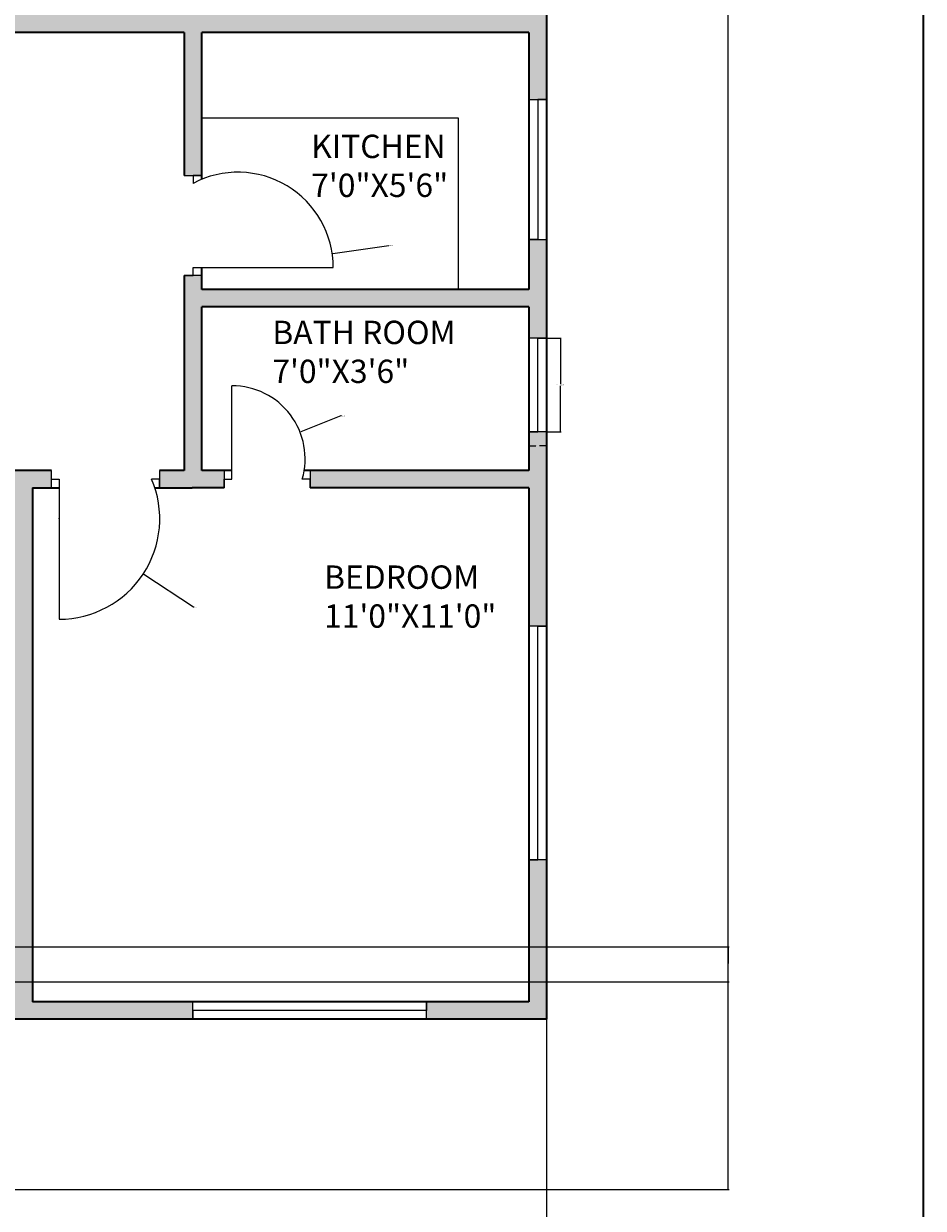
# Model space of a CAD drawing. Units: inches. Extents: x 2314 to 3223, y 1382 to 2735.
# Tile 5 of 14: x 2992 to 3223, y 1560 to 1864. Entities that reach past the tile are written whole.
import ezdxf

# ---------------------------------------------------------------- set-up
doc = ezdxf.new("R2010")
doc.units = ezdxf.units.IN
for name, color, linetype, lineweight in [('A-ANNO-DIMS', 2, 'Continuous', 18), ('A-ANNO-TTLB', 7, 'Continuous', 35), ('A-AREA-IDEN', 7, 'Continuous', 18), ('A-DOOR', 3, 'Continuous', 18), ('A-FLOR-FIXT', 8, 'Continuous', 18), ('A-GLAZ', 4, 'Continuous', 18), ('A-WALL', 7, 'Continuous', 35)]:
    doc.layers.add(name, color=color, linetype=linetype, lineweight=lineweight)
doc.layers.add('A-WALL-PATT', color=251, linetype='Continuous', lineweight=13, true_color=0x636466)
doc.styles.get("Standard").update_dxf_attribs({"font": 'arial.ttf'})
doc.dimstyles.get("Standard").update_dxf_attribs({"dimtxt": 0.18, "dimasz": 0.18, "dimexe": 0.18, "dimexo": 0.0625, "dimgap": 0.09, "dimtad": 0, "dimtih": 1, "dimtoh": 1, "dimdec": 4, "dimzin": 0, "dimdsep": 46, "dimtxsty": 'Standard', "dimcen": 0.09, "dimadec": 0, "dimazin": 0, "dimtfac": 1, "dimtdec": 4, "dimtofl": 0, "dimtmove": 0, "dimatfit": 3, "dimfxl": 1, "dimtolj": 1, "dimtzin": 0, "dimarcsym": 0})

# ---------------------------------------------------------------- blocks, each defined once
blk = doc.blocks.new('WIN-PLAN-24')
for p, q in [((0, 24), (4.5, 24)), ((4.5, 24), (2.25, 24)), ((2.25, 24), (2.25, 0)), ((2.25, 0), (0, 0)), ((0, 0), (4.5, 0))]:
    blk.add_line(p, q)
blk = doc.blocks.new('WIN-PLAN-60')
for p, q in [((0, 4.5), (0, 0)), ((60, 2.25), (60, 4.5)), ((60, 4.5), (60, 0)), ((0, 0), (0, 2.25)), ((0, 2.25), (60, 2.25))]:
    blk.add_line(p, q)
blk = doc.blocks.new('WIN-PLAN-36')
for p, q in [((0, 36), (4.5, 36)), ((4.5, 36), (2.25, 36)), ((2.25, 36), (2.25, 0)), ((2.25, 0), (0, 0)), ((0, 0), (4.5, 0))]:
    blk.add_line(p, q)
blk = doc.blocks.new('*D13')
at = {"layer": 'A-ANNO-DIMS', "color": 0, "lineweight": -2, "transparency": 16777216}
for p, q in [((3125.96, 1783.31), (3129.67, 1783.31)), ((3129.49, 1783.13), (3129.49, 1771.49)), ((3129.49, 1759.49), (3129.49, 1771.13)), ((3125.96, 1759.31), (3129.67, 1759.31))]:
    blk.add_line(p, q, dxfattribs=at)
at = {"layer": 'A-ANNO-DIMS', "color": 0, "transparency": 16777216}
for points in [[(3129.46, 1783.13), (3129.52, 1783.13), (3129.49, 1783.31)], [(3129.46, 1759.49), (3129.52, 1759.49), (3129.49, 1759.31)]]:
    blk.add_solid(points, dxfattribs=at)
at = {"layer": 'Defpoints', "color": 0, "transparency": 16777216}
for p in [(3125.89, 1783.31), (3125.89, 1759.31), (3129.49, 1759.31)]:
    blk.add_point(p, dxfattribs=at)
at = {"layer": 'A-ANNO-DIMS', "color": 0, "transparency": 16777216, "insert": (3129.49, 1771.31), "char_height": 0.18, "attachment_point": 5}
blk.add_mtext('\\A1;WINDOW 24 TYP.', dxfattribs=at)
blk = doc.blocks.new('*D14')
at = {"layer": 'A-ANNO-DIMS', "color": 0, "lineweight": -2, "transparency": 16777216}
for p, q in [((3121.39, 1759.25), (3121.39, 1755.53)), ((3125.89, 1759.25), (3125.89, 1755.53)), ((3121.57, 1755.71), (3123.18, 1755.71)), ((3125.71, 1755.71), (3124.1, 1755.71))]:
    blk.add_line(p, q, dxfattribs=at)
at = {"layer": 'A-ANNO-DIMS', "color": 0, "transparency": 16777216}
for points in [[(3121.57, 1755.74), (3121.57, 1755.68), (3121.39, 1755.71)], [(3125.71, 1755.74), (3125.71, 1755.68), (3125.89, 1755.71)]]:
    blk.add_solid(points, dxfattribs=at)
at = {"layer": 'Defpoints', "color": 0, "transparency": 16777216}
for p in [(3121.39, 1759.31), (3125.89, 1759.31), (3121.39, 1755.71)]:
    blk.add_point(p, dxfattribs=at)
at = {"layer": 'A-ANNO-DIMS', "color": 0, "transparency": 16777216, "insert": (3123.64, 1755.71), "char_height": 0.18, "attachment_point": 5}
blk.add_mtext('\\A1;5 TYP.', dxfattribs=at)
blk = doc.blocks.new('*D29')
at = {"layer": 'A-ANNO-DIMS', "color": 0, "lineweight": -2, "transparency": 16777216}
for p, q in [((2410.39, 1608.32), (2410.39, 1434.13)), ((3125.89, 1608.32), (3125.89, 1434.13)), ((2410.57, 1434.31), (2767.75, 1434.31)), ((3125.71, 1434.31), (2768.54, 1434.31))]:
    blk.add_line(p, q, dxfattribs=at)
at = {"layer": 'A-ANNO-DIMS', "color": 0, "transparency": 16777216}
for points in [[(2410.57, 1434.34), (2410.57, 1434.28), (2410.39, 1434.31)], [(3125.71, 1434.34), (3125.71, 1434.28), (3125.89, 1434.31)]]:
    blk.add_solid(points, dxfattribs=at)
at = {"layer": 'Defpoints', "color": 0, "transparency": 16777216}
for p in [(2410.39, 1608.38), (3125.89, 1608.38), (3125.89, 1434.31)]:
    blk.add_point(p, dxfattribs=at)
at = {"layer": 'A-ANNO-DIMS', "color": 0, "transparency": 16777216, "insert": (2768.14, 1434.31), "char_height": 0.18, "attachment_point": 5}
blk.add_mtext('\\A1;715.5', dxfattribs=at)
blk = doc.blocks.new('*D30')
at = {"layer": 'A-ANNO-DIMS', "color": 0, "lineweight": -2, "transparency": 16777216}
for p, q in [((3125.96, 2381.78), (3172.77, 2381.78)), ((3172.59, 2381.6), (3172.59, 1973.38)), ((3172.59, 1564.8), (3172.59, 1973.02)), ((2822.96, 1564.62), (3172.77, 1564.62))]:
    blk.add_line(p, q, dxfattribs=at)
at = {"layer": 'A-ANNO-DIMS', "color": 0, "transparency": 16777216}
for points in [[(3172.56, 2381.6), (3172.62, 2381.6), (3172.59, 2381.78)], [(3172.56, 1564.8), (3172.62, 1564.8), (3172.59, 1564.62)]]:
    blk.add_solid(points, dxfattribs=at)
at = {"layer": 'Defpoints', "color": 0, "transparency": 16777216}
for p in [(3125.89, 2381.78), (2822.89, 1564.62), (3172.59, 1564.62)]:
    blk.add_point(p, dxfattribs=at)
at = {"layer": 'A-ANNO-DIMS', "color": 0, "transparency": 16777216, "insert": (3172.59, 1973.2), "char_height": 0.18, "attachment_point": 5}
blk.add_mtext('\\A1;817.2', dxfattribs=at)
blk = doc.blocks.new('*D38')
at = {"layer": 'A-ANNO-DIMS', "color": 0, "lineweight": -2, "transparency": 16777216}
for p, q in [((2818.46, 1627), (3172.77, 1627)), ((3172.59, 1626.82), (3172.59, 1622.68)), ((3172.59, 1618.18), (3172.59, 1622.32)), ((2818.46, 1618), (3172.77, 1618))]:
    blk.add_line(p, q, dxfattribs=at)
at = {"layer": 'A-ANNO-DIMS', "color": 0, "transparency": 16777216}
for points in [[(3172.56, 1626.82), (3172.62, 1626.82), (3172.59, 1627)], [(3172.56, 1618.18), (3172.62, 1618.18), (3172.59, 1618)]]:
    blk.add_solid(points, dxfattribs=at)
at = {"layer": 'Defpoints', "color": 0, "transparency": 16777216}
for p in [(2818.39, 1627), (3172.59, 1627), (2818.39, 1618)]:
    blk.add_point(p, dxfattribs=at)
at = {"layer": 'A-ANNO-DIMS', "color": 0, "transparency": 16777216, "insert": (3172.59, 1622.5), "char_height": 0.18, "attachment_point": 5}
blk.add_mtext('\\A1;9', dxfattribs=at)
blk = doc.blocks.new('*D80')
at = {"layer": 'A-ANNO-DIMS', "color": 0, "lineweight": -2, "transparency": 16777216}
for p, q in [((3000.65, 1736.98), (3000.83, 1736.98)), ((3000.74, 1736.89), (3000.74, 1737.07)), ((3035.25, 1714.2), (3022.46, 1722.64)), ((3035.43, 1714.2), (3035.25, 1714.2))]:
    blk.add_line(p, q, dxfattribs=at)
at = {"layer": 'A-ANNO-DIMS', "color": 0, "transparency": 16777216}
blk.add_solid([(3022.48, 1722.67), (3022.44, 1722.62), (3022.31, 1722.74)], dxfattribs=at)
at = {"layer": 'Defpoints', "color": 0, "transparency": 16777216}
for p in [(3000.74, 1736.98), (3022.31, 1722.74)]:
    blk.add_point(p, dxfattribs=at)
at = {"layer": 'A-ANNO-DIMS', "color": 0, "transparency": 16777216, "insert": (3035.91, 1714.2), "char_height": 0.18, "attachment_point": 5}
blk.add_mtext('\\A1;R25.84', dxfattribs=at)
blk = doc.blocks.new('*D83')
at = {"layer": 'A-ANNO-DIMS', "color": 0, "lineweight": -2, "transparency": 16777216}
for p, q in [((3085.44, 1807.09), (3071.07, 1805.01)), ((3046.56, 1801.48), (3046.74, 1801.48)), ((3046.65, 1801.39), (3046.65, 1801.57))]:
    blk.add_line(p, q, dxfattribs=at)
at = {"layer": 'A-ANNO-DIMS', "color": 0, "transparency": 16777216}
blk.add_solid([(3071.06, 1805.04), (3071.07, 1804.98), (3070.89, 1804.98)], dxfattribs=at)
at = {"layer": 'Defpoints', "color": 0, "transparency": 16777216}
for p in [(3070.89, 1804.98), (3046.65, 1801.48)]:
    blk.add_point(p, dxfattribs=at)
at = {"layer": 'A-ANNO-DIMS', "color": 0, "transparency": 16777216, "insert": (3085.99, 1807.09), "char_height": 0.18, "attachment_point": 5}
blk.add_mtext('\\A1;R24.496', dxfattribs=at)
blk = doc.blocks.new('*D95')
at = {"layer": 'A-ANNO-DIMS', "color": 0, "lineweight": -2, "transparency": 16777216}
for p, q in [((3073.1, 1763.38), (3062.78, 1759.31)), ((3073.28, 1763.38), (3073.1, 1763.38)), ((3045.04, 1752.34), (3045.22, 1752.34)), ((3045.13, 1752.25), (3045.13, 1752.43))]:
    blk.add_line(p, q, dxfattribs=at)
at = {"layer": 'A-ANNO-DIMS', "color": 0, "transparency": 16777216}
blk.add_solid([(3062.77, 1759.33), (3062.79, 1759.28), (3062.61, 1759.24)], dxfattribs=at)
at = {"layer": 'Defpoints', "color": 0, "transparency": 16777216}
for p in [(3062.61, 1759.24), (3045.13, 1752.34)]:
    blk.add_point(p, dxfattribs=at)
at = {"layer": 'A-ANNO-DIMS', "color": 0, "transparency": 16777216, "insert": (3073.76, 1763.38), "char_height": 0.18, "attachment_point": 5}
blk.add_mtext('\\A1;R18.79', dxfattribs=at)

msp = doc.modelspace()

# ---------------------------------------------------------------- hatches: boundary and pattern name
at = {"layer": 'A-WALL-PATT'}
h = msp.add_hatch(color=256, dxfattribs=at)
h.dxf.hatch_style = 1
h.paths.add_polyline_path([(2443.3302, 2379.5332), (2443.3302, 2381.7832), (2410.3927, 2381.7832), (2410.3927, 2336.7008), (2414.8927, 2336.7008), (2414.8927, 2377.2832), (2443.3302, 2377.2832)])
h.paths.add_polyline_path([(2561.3645, 2379.5332), (2561.3645, 2381.7832), (2503.3302, 2381.7832), (2503.3302, 2377.2832), (2546.8927, 2377.2832), (2546.8927, 2245.2832), (2541.8787, 2245.2832), (2541.8787, 2240.7832), (2551.3927, 2240.7832), (2551.3927, 2377.2832), (2561.3645, 2377.2832)])
h.paths.add_polyline_path([(2656.0607, 2381.7832), (2597.3645, 2381.7832), (2597.3645, 2377.2832), (2617.3927, 2377.2832), (2617.3927, 2257.2832), (2584.2532, 2257.2832), (2584.2532, 2252.7832), (2625.8528, 2252.7832), (2625.8528, 2255.0332), (2625.8528, 2257.2832), (2621.8927, 2257.2832), (2621.8927, 2377.2832), (2656.0607, 2377.2832), (2656.0607, 2379.5332)])
h.paths.add_polyline_path([(2807.3418, 2381.7832), (2716.0607, 2381.7832), (2716.0607, 2377.2832), (2765.8927, 2377.2832), (2765.8927, 2257.2832), (2661.6935, 2257.2832), (2661.6935, 2252.7832), (2765.8927, 2252.7832), (2765.8927, 2146.2832), (2760.9259, 2146.2832), (2760.9259, 2141.8832), (2775.7119, 2141.8832), (2775.7119, 2146.2832), (2770.3927, 2146.2832), (2770.3927, 2252.7832), (2877.684, 2252.7832), (2877.684, 2255.0332), (2877.684, 2257.2832), (2770.3927, 2257.2832), (2770.3927, 2377.2832), (2807.3418, 2377.2832), (2807.3418, 2379.5332)])
h.paths.add_polyline_path([(2937.2118, 2381.7832), (2867.3418, 2381.7832), (2867.3418, 2377.2832), (2914.3927, 2377.2832), (2914.3927, 2257.2832), (2908.4124, 2257.2832), (2908.4124, 2252.7832), (2960.6432, 2252.7832), (2960.6432, 2255.0332), (2960.6432, 2257.2832), (2918.8927, 2257.2832), (2918.8927, 2377.2832), (2937.2118, 2377.2832)])
h.paths.add_polyline_path([(3022.1601, 2381.7832), (2973.2118, 2381.7832), (2973.2118, 2379.5332), (2973.2118, 2377.2832), (2984.8927, 2377.2832), (2984.8927, 2257.2832), (2980.0601, 2257.2832), (2980.0601, 2252.7832), (2984.8927, 2252.7832), (2984.8927, 2240.7832), (2995.668, 2240.7832), (2995.668, 2243.0332), (2995.668, 2245.2832), (2989.3927, 2245.2832), (2989.3927, 2377.2832), (3022.1601, 2377.2832), (3022.1601, 2379.5332)])
h.paths.add_polyline_path([(3125.8927, 2381.7832), (3082.1601, 2381.7832), (3082.1601, 2377.2832), (3121.3927, 2377.2832), (3121.3927, 2334.7388), (3125.8927, 2334.7388)])
h.paths.add_polyline_path([(3125.8927, 2274.7388), (3121.3927, 2274.7388), (3121.3927, 2245.2832), (3066.4832, 2245.2832), (3066.4832, 2240.7832), (3121.3927, 2240.7832), (3121.3927, 2232.1868), (3125.8927, 2232.1868)])
h.paths.add_polyline_path([(3125.8927, 2208.1868), (3121.3927, 2208.1868), (3121.3927, 2198.7832), (3037.3927, 2198.7832), (3037.3927, 2240.7832), (3041.2694, 2240.7832), (3041.2694, 2243.0332), (3041.2694, 2245.2832), (3026.8205, 2245.2832), (3026.8205, 2240.7832), (3032.8927, 2240.7832), (3032.8927, 2190.4022), (3037.3927, 2190.4022), (3037.3927, 2194.2832), (3121.3927, 2194.2832), (3121.3927, 2182.1835), (3125.8927, 2182.1835)])
h.paths.add_polyline_path([(3125.8927, 2158.1835), (3121.3927, 2158.1835), (3121.3927, 2146.2832), (3037.3927, 2146.2832), (3037.3927, 2169.3726), (3035.1427, 2169.3726), (3032.8927, 2169.3726), (3032.8927, 2146.2832), (2812.7301, 2146.2832), (2812.7301, 2144.0832), (2812.7301, 2141.8832), (2818.3927, 2141.8832), (2818.3927, 1970.1316), (2822.8927, 1970.1316), (2822.8927, 1978.8832), (2903.9846, 1978.8832), (2903.9846, 1981.1332), (2903.9846, 1983.3832), (2822.8927, 1983.3832), (2822.8927, 2115.3832), (2851.7162, 2115.3832), (2851.7162, 2117.6332), (2851.7162, 2119.8832), (2822.8927, 2119.8832), (2822.8927, 2141.8832), (3125.8927, 2141.8832)])
h.paths.add_polyline_path([(3125.8927, 2119.8832), (3081.193, 2119.8832), (3081.193, 2115.3832), (3121.3927, 2115.3832), (3121.3927, 2071.8188), (3125.8927, 2071.8188)], flags=17)
h.paths.add_polyline_path([(2989.3927, 2115.3832), (3021.193, 2115.3832), (3021.193, 2117.6332), (3021.193, 2119.8832), (2979.123, 2119.8832), (2979.123, 2115.3832), (2984.8927, 2115.3832), (2984.8927, 2019.3832), (2981.9225, 2019.3832), (2981.9225, 2014.8832), (2984.8927, 2014.8832), (2984.8927, 1983.3832), (2984.8927, 1978.8832), (2989.3927, 1978.8832), (2989.3927, 1983.3832)], flags=17)
h.paths.add_polyline_path([(2947.3927, 2115.3832), (2955.123, 2115.3832), (2955.123, 2117.6332), (2955.123, 2119.8832), (2911.7162, 2119.8832), (2911.7162, 2115.3832), (2942.8927, 2115.3832), (2942.8927, 1983.3832), (2936.7017, 1983.3832), (2936.7017, 1978.8832), (2947.3927, 1978.8832), (2947.3927, 1983.3832), (2947.3927, 2014.8832), (2960.7167, 2014.8832), (2960.7167, 2017.1332), (2960.7167, 2019.3832), (2947.3927, 2019.3832)], flags=17)
h.paths.add_polyline_path([(3037.3927, 1978.8832), (3041.8276, 1978.8832), (3041.8276, 1981.1332), (3041.8276, 1983.3832), (3025.477, 1983.3832), (3025.477, 1978.8832), (3032.8927, 1978.8832), (3032.8927, 1927.1259), (3035.1427, 1927.1259), (3037.3927, 1927.1259)])
h.paths.add_polyline_path([(3125.8927, 2011.8188), (3123.6427, 2011.8188), (3121.3927, 2011.8188), (3121.3927, 1983.3832), (3065, 1983.3832), (3065, 1978.8832), (3121.3927, 1978.8832), (3121.3927, 1970.5932), (3125.8927, 1970.5932)], flags=17)
h.paths.add_polyline_path([(2994.2341, 1983.3832), (2989.3927, 1983.3832), (2989.3927, 1978.8832), (2994.2341, 1978.8832), (2994.2341, 1981.1332)], flags=16)
h.paths.add_polyline_path([(3125.8927, 1946.5932), (3121.3927, 1946.5932), (3121.3927, 1936.8832), (3037.3927, 1936.8832), (3037.3927, 1932.3832), (3121.3927, 1932.3832), (3121.3927, 1919.825), (3125.8927, 1919.825)])
h.paths.add_polyline_path([(3125.8927, 1883.825), (3121.3927, 1883.825), (3121.3927, 1866.3832), (3037.3927, 1866.3832), (3037.3927, 1899.0954), (3035.1427, 1899.0954), (3032.8927, 1899.0954), (3032.8927, 1866.3832), (2822.8927, 1866.3832), (2822.8927, 1938.7212), (2820.6427, 1938.7212), (2818.3927, 1938.7212), (2818.3927, 1786.9239), (2822.8927, 1786.9239), (2822.8927, 1861.8832), (3032.8927, 1861.8832), (3032.8927, 1825.1023), (3037.3927, 1825.1023), (3037.3927, 1861.8832), (3121.3927, 1861.8832), (3121.3927, 1844.6765), (3125.8927, 1844.6765)])
h.paths.add_polyline_path([(3125.8927, 1808.6765), (3121.3927, 1808.6765), (3121.3927, 1795.8832), (3037.3927, 1795.8832), (3037.3927, 1799.4755), (3032.8927, 1799.4755), (3032.8927, 1749.3832), (3026.5034, 1749.3832), (3026.5034, 1744.8832), (3032.8927, 1744.8832), (3034.9255, 1744.8832), (3043.1326, 1744.8832), (3043.1326, 1747.1332), (3043.1326, 1749.3832), (3037.3927, 1749.3832), (3037.3927, 1791.3832), (3121.3927, 1791.3832), (3121.3927, 1783.3103), (3125.8927, 1783.3103)])
h.paths.add_polyline_path([(3125.8927, 1759.3103), (3121.3927, 1759.3103), (3121.3927, 1749.3832), (3065.1845, 1749.3832), (3065.1845, 1744.8832), (3121.3927, 1744.8832), (3121.3927, 1709.3573), (3125.8927, 1709.3573)])
h.paths.add_polyline_path([(3125.8927, 1649.3573), (3121.3927, 1649.3573), (3121.3927, 1612.8832), (3095.116, 1612.8832), (3095.116, 1608.3832), (3125.8927, 1608.3832)])
h.paths.add_polyline_path([(3035.116, 1612.8832), (2993.8927, 1612.8832), (2993.8927, 1744.8832), (2998.7409, 1744.8832), (2998.7409, 1749.3832), (2989.3927, 1749.3832), (2989.3927, 1744.8832), (2989.3927, 1701.3832), (2972.8226, 1701.3832), (2972.8226, 1696.8832), (2989.3927, 1696.8832), (2989.3927, 1612.8832), (2978.2225, 1612.8832), (2978.2225, 1608.3832), (3035.116, 1608.3832), (3035.116, 1610.6332)])
h.paths.add_polyline_path([(2947.3927, 1696.8832), (2950.7566, 1696.8832), (2950.7566, 1699.1332), (2950.7566, 1701.3832), (2947.3927, 1701.3832), (2947.3927, 1744.8832), (2947.3927, 1749.3832), (2937.649, 1749.3832), (2937.649, 1744.8832), (2942.8927, 1744.8832), (2942.8927, 1612.8832), (2907.783, 1612.8832), (2907.783, 1608.3832), (2954.2225, 1608.3832), (2954.2225, 1610.6332), (2954.2225, 1612.8832), (2947.3927, 1612.8832)])
h.paths.add_polyline_path([(2822.8927, 1744.8832), (2905.3491, 1744.8832), (2905.3491, 1747.1332), (2905.3491, 1749.3832), (2822.8927, 1749.3832), (2822.8927, 1756.9185), (2818.3927, 1756.9185), (2818.3927, 1612.8832), (2818.3927, 1569.1205), (2722.3927, 1569.1205), (2722.3927, 1612.8832), (2722.3927, 1756.9185), (2717.8927, 1756.9185), (2717.8927, 1750.0143), (2633.6297, 1750.0143), (2633.6437, 1745.2665), (2717.8927, 1745.5143), (2717.8927, 1612.8832), (2689.8467, 1612.8832), (2689.8467, 1608.3832), (2717.8927, 1608.3832), (2717.8927, 1564.6205), (2722.3927, 1564.6205), (2822.8927, 1564.6205), (2822.8927, 1569.1205), (2822.8927, 1608.3832), (2847.783, 1608.3832), (2847.783, 1610.6332), (2847.783, 1612.8832), (2822.8927, 1612.8832)])
h.paths.add_polyline_path([(2629.8467, 1612.8832), (2597.8927, 1612.8832), (2597.8927, 1744.8832), (2597.8927, 1745.1613), (2601.5887, 1745.1721), (2601.5816, 1747.5932), (2601.5745, 1750.0143), (2593.3927, 1750.0143), (2593.3927, 1744.8832), (2593.3927, 1713.3832), (2589.7588, 1713.3832), (2589.7588, 1708.8832), (2593.3927, 1708.8832), (2593.3927, 1612.8832), (2582.3793, 1612.8832), (2582.3793, 1608.3832), (2629.8467, 1608.3832), (2629.8467, 1610.6332)])
h.paths.add_polyline_path([(2551.3927, 1708.8832), (2567.6776, 1708.8832), (2567.6776, 1711.1332), (2567.6776, 1713.3832), (2551.3927, 1713.3832), (2551.3927, 1744.8832), (2551.3927, 1750.0143), (2543.5657, 1750.0143), (2543.5657, 1747.5079), (2543.5657, 1745.0014), (2546.8927, 1745.0112), (2546.8927, 1744.8832), (2546.8927, 1612.8832), (2502.9339, 1612.8832), (2502.9339, 1608.3832), (2558.3793, 1608.3832), (2558.3793, 1610.6332), (2558.3793, 1612.8832), (2551.3927, 1612.8832)])
h.paths.add_polyline_path([(2414.8927, 1656.2547), (2410.3927, 1656.2547), (2410.3927, 1608.3832), (2442.9339, 1608.3832), (2442.9339, 1610.6332), (2442.9339, 1612.8832), (2414.8927, 1612.8832)])
h.paths.add_polyline_path([(2414.8927, 1744.8832), (2468.8906, 1744.8832), (2468.8906, 1747.1332), (2468.8906, 1749.3832), (2414.8927, 1749.3832), (2414.8927, 1757.7622), (2410.3927, 1757.7622), (2410.3927, 1716.2547), (2414.8927, 1716.2547)])
h.paths.add_polyline_path([(2414.8927, 1791.3832), (2498.8927, 1791.3832), (2498.8927, 1749.3832), (2492.9799, 1749.3832), (2492.9799, 1744.8832), (2498.8927, 1744.8832), (2503.3927, 1744.8832), (2508.0135, 1744.8968), (2508.0059, 1747.4556), (2507.9984, 1750.0143), (2503.3927, 1750.0143), (2503.3927, 1802.6362), (2501.1427, 1802.6362), (2498.8927, 1802.6362), (2498.8927, 1795.8832), (2414.8927, 1795.8832), (2414.8927, 1808.0943), (2410.3927, 1808.0943), (2410.3927, 1781.7622), (2414.8927, 1781.7622)])
h.paths.add_polyline_path([(2722.3927, 1937.589), (2720.1427, 1937.589), (2717.8927, 1937.589), (2717.8927, 1866.3832), (2503.3927, 1866.3832), (2503.3927, 1896.3484), (2498.8927, 1896.3484), (2498.8927, 1866.3832), (2414.8927, 1866.3832), (2414.8927, 1882.1496), (2410.3927, 1882.1496), (2410.3927, 1844.0943), (2414.8927, 1844.0943), (2414.8927, 1861.8832), (2498.8927, 1861.8832), (2498.8927, 1831.4783), (2501.1427, 1831.4783), (2503.3927, 1831.4783), (2503.3927, 1861.8832), (2717.8927, 1861.8832), (2717.8927, 1786.9239), (2722.3927, 1786.9239)])
h.paths.add_polyline_path([(2414.8927, 1932.3832), (2498.8927, 1932.3832), (2498.8927, 1924.7883), (2503.3927, 1924.7883), (2503.3927, 1978.8832), (2505.8599, 1978.8832), (2505.8599, 1981.1332), (2505.8599, 1983.3832), (2493.3697, 1983.3832), (2493.3697, 1978.8832), (2498.8927, 1978.8832), (2498.8927, 1936.8832), (2414.8927, 1936.8832), (2414.8927, 1943.2834), (2410.3927, 1943.2834), (2410.3927, 1918.1496), (2414.8927, 1918.1496)])
h.paths.add_polyline_path([(2414.8927, 2020.3133), (2412.6427, 2020.3133), (2410.3927, 2020.3133), (2410.3927, 1967.2834), (2414.8927, 1967.2834), (2414.8927, 1978.8832), (2468.8513, 1978.8832), (2468.8513, 1981.1332), (2468.8513, 1983.3832), (2414.8927, 1983.3832)])
h.paths.add_polyline_path([(2414.8927, 2115.3832), (2453.004, 2115.3832), (2453.004, 2117.6332), (2453.004, 2119.8832), (2410.3927, 2119.8832), (2410.3927, 2080.3133), (2414.8927, 2080.3133)], flags=17)
h.paths.add_polyline_path([(2559.0969, 2117.6332), (2559.0969, 2119.8832), (2513.004, 2119.8832), (2513.004, 2115.3832), (2546.8927, 2115.3832), (2546.8927, 1983.3832), (2542.7531, 1983.3832), (2542.7531, 1978.8832), (2551.3927, 1978.8832), (2551.3927, 2014.8832), (2570.3098, 2014.8832), (2570.3098, 2017.1332), (2570.3098, 2019.3832), (2551.3927, 2019.3832), (2551.3927, 2115.3832), (2559.0969, 2115.3832)], flags=17)
h.paths.add_polyline_path([(2628.5073, 2117.6332), (2628.5073, 2119.8832), (2583.0969, 2119.8832), (2583.0969, 2115.3832), (2593.3927, 2115.3832), (2593.3927, 2019.3832), (2590.2108, 2019.3832), (2590.2108, 2014.8832), (2593.3927, 2014.8832), (2593.3927, 1978.8832), (2601.5907, 1978.8832), (2601.5907, 1981.1332), (2601.5907, 1983.3832), (2597.8927, 1983.3832), (2597.8927, 2115.3832), (2628.5073, 2115.3832)], flags=17)
h.paths.add_polyline_path([(2722.3927, 2141.8832), (2726.9871, 2141.8832), (2726.9871, 2144.2705), (2726.9871, 2146.2832), (2503.3927, 2146.2832), (2503.3927, 2168.2161), (2501.1427, 2168.2161), (2498.8927, 2168.2161), (2498.8927, 2146.2832), (2414.8927, 2146.2832), (2414.8927, 2156.5041), (2410.3927, 2156.5041), (2410.3927, 2141.8832), (2717.8927, 2141.8832), (2717.8927, 2119.8832), (2688.5073, 2119.8832), (2688.5073, 2115.3832), (2717.8927, 2115.3832), (2717.8927, 1983.3832), (2633.2454, 1983.3832), (2633.2454, 1978.8832), (2717.8927, 1978.8832), (2717.8927, 1970.1316), (2720.1427, 1970.1316), (2722.3927, 1970.1316)])
h.paths.add_polyline_path([(2557.3704, 1462.9278), (2940.0934, 1462.9278), (2940.0934, 1512.3848), (2557.3704, 1512.3848)], flags=9)
h.paths.add_polyline_path([(2846.2527, 1703.1384), (2892.8612, 1703.1384), (2892.8612, 1725.5272), (2846.2527, 1725.5272)], flags=25)
h.paths.add_polyline_path([(2885.6102, 1812.1147), (2946.1505, 1812.1147), (2946.1505, 1834.5035), (2885.6102, 1834.5035)], flags=25)
h.paths.add_polyline_path([(2885.6102, 1884.183), (2946.1505, 1884.183), (2946.1505, 1906.5718), (2885.6102, 1906.5718)], flags=25)
h.paths.add_polyline_path([(3066.365, 1705.5431), (3112.9735, 1705.5431), (3112.9735, 1727.9319), (3066.365, 1727.9319)], flags=9)
h.paths.add_polyline_path([(3061.8255, 1887.7513), (3101.6154, 1887.7513), (3101.6154, 1910.1401), (3061.8255, 1910.1401)], flags=25)
h.paths.add_polyline_path([(3063.3679, 1816.2121), (3103.1578, 1816.2121), (3103.1578, 1838.6009), (3063.3679, 1838.6009)], flags=25)
h.paths.add_polyline_path([(3053.3743, 1768.416), (3107.1329, 1768.416), (3107.1329, 1790.8048), (3053.3743, 1790.8048)], flags=25)
h.paths.add_polyline_path([(3061.6068, 1943.822), (3115.3653, 1943.822), (3115.3653, 1966.2109), (3061.6068, 1966.2109)], flags=9)
h.paths.add_polyline_path([(2745.0978, 1763.6604), (2797.9354, 1763.6604), (2797.9354, 1776.0247), (2745.0978, 1776.0247)], flags=9)
h.paths.add_polyline_path([(2574.2135, 1819.2586), (2634.7538, 1819.2586), (2634.7538, 1841.6474), (2574.2135, 1841.6474)], flags=25)
h.paths.add_polyline_path([(2574.2135, 1891.3269), (2634.7538, 1891.3269), (2634.7538, 1913.7157), (2574.2135, 1913.7157)], flags=25)
h.paths.add_polyline_path([(2638.4466, 1702.43), (2685.0551, 1702.43), (2685.0551, 1724.8188), (2638.4466, 1724.8188)], flags=25)
h.paths.add_polyline_path([(2435.9715, 1697.1215), (2482.5799, 1697.1215), (2482.5799, 1719.5103), (2435.9715, 1719.5103)], flags=9)
h.paths.add_polyline_path([(2431.2046, 1893.7833), (2470.9945, 1893.7833), (2470.9945, 1916.1721), (2431.2046, 1916.1721)], flags=25)
h.paths.add_polyline_path([(2439.8144, 1817.2116), (2479.6043, 1817.2116), (2479.6043, 1839.6004), (2439.8144, 1839.6004)], flags=25)
h.paths.add_polyline_path([(2441.2607, 1753.0942), (2495.0192, 1753.0942), (2495.0192, 1775.483), (2441.2607, 1775.483)], flags=25)
h.paths.add_polyline_path([(2421.216, 1945.3109), (2474.9746, 1945.3109), (2474.9746, 1967.6997), (2421.216, 1967.6997)], flags=25)
h.paths.add_polyline_path([(2585.4464, 1627.5703), (2585.4464, 1679), (2563.0576, 1679), (2563.0576, 1627.5703)], flags=9)
h.paths.add_polyline_path([(2978.3497, 1618.7039), (2978.3497, 1670.1337), (2955.9609, 1670.1337), (2955.9609, 1618.7039)], flags=9)
h.paths.add_polyline_path([(2975.9502, 2041.7828), (2975.9502, 2093.2125), (2953.5614, 2093.2125), (2953.5614, 2041.7828)], flags=25)
h.paths.add_polyline_path([(2835.6537, 1989.2068), (2882.2621, 1989.2068), (2882.2621, 2011.5956), (2835.6537, 2011.5956)], flags=25)
h.paths.add_polyline_path([(2649.3769, 1997.5659), (2695.9853, 1997.5659), (2695.9853, 2019.9547), (2649.3769, 2019.9547)], flags=25)
h.paths.add_polyline_path([(2579.9087, 2040.3429), (2579.9087, 2091.7726), (2557.5198, 2091.7726), (2557.5198, 2040.3429)], flags=25)
h.paths.add_polyline_path([(2783.2404, 1883.1956), (2783.2404, 2067.1369), (2764.694, 2067.1369), (2764.694, 1883.1956)], flags=9)
h.paths.add_polyline_path([(3055.8435, 1993.5571), (3102.4519, 1993.5571), (3102.4519, 2015.9459), (3055.8435, 2015.9459)], flags=25)
h.paths.add_polyline_path([(2423.6009, 1984.6082), (2470.2094, 1984.6082), (2470.2094, 2006.997), (2423.6009, 2006.997)], flags=25)
h.paths.add_polyline_path([(2973.4115, 2123.1668), (3013.1319, 2123.1668), (3013.1319, 2135.531), (2973.4115, 2135.531)], flags=25)
h.paths.add_polyline_path([(2534.3846, 2124.6231), (2574.105, 2124.6231), (2574.105, 2136.9874), (2534.3846, 2136.9874)], flags=25)
h.paths.add_polyline_path([(2829.1368, 2188.1931), (2889.411, 2188.1931), (2889.411, 2210.5819), (2829.1368, 2210.5819)], flags=9)
h.paths.add_polyline_path([(2633.2547, 2185.0437), (2693.5289, 2185.0437), (2693.5289, 2207.4325), (2633.2547, 2207.4325)], flags=9)
h.paths.add_polyline_path([(2445.1812, 2167.0395), (2496.611, 2167.0395), (2496.611, 2189.4284), (2445.1812, 2189.4284)], flags=9)
h.paths.add_polyline_path([(2429.1678, 2194.5482), (2480.5975, 2194.5482), (2480.5975, 2216.937), (2429.1678, 2216.937)], flags=9)
h.paths.add_polyline_path([(3060.1138, 2158.1056), (3111.5436, 2158.1056), (3111.5436, 2180.4944), (3060.1138, 2180.4944)], flags=9)
h.paths.add_polyline_path([(3055.6824, 2201.2631), (3107.1122, 2201.2631), (3107.1122, 2223.652), (3055.6824, 2223.652)], flags=25)
h.paths.add_polyline_path([(3044.3482, 2257.7345), (3090.9567, 2257.7345), (3090.9567, 2280.1233), (3044.3482, 2280.1233)], flags=9)
h.paths.add_polyline_path([(2942.5437, 2306.9625), (2982.3336, 2306.9625), (2982.3336, 2329.3513), (2942.5437, 2329.3513)], flags=9)
h.paths.add_polyline_path([(2799.5865, 2259.1663), (2846.195, 2259.1663), (2846.195, 2281.5551), (2799.5865, 2281.5551)], flags=25)
h.paths.add_polyline_path([(2670.4998, 2261.1493), (2717.1082, 2261.1493), (2717.1082, 2283.5381), (2670.4998, 2283.5381)], flags=25)
h.paths.add_polyline_path([(2553.0333, 2302.7735), (2592.8232, 2302.7735), (2592.8232, 2325.1624), (2553.0333, 2325.1624)], flags=9)
h.paths.add_polyline_path([(2432.0288, 2268.6489), (2478.6372, 2268.6489), (2478.6372, 2291.0377), (2432.0288, 2291.0377)], flags=9)
h = msp.add_hatch(color=256, dxfattribs=at)
h.dxf.hatch_style = 1
h.paths.add_polyline_path([(2503.3927, 2240.7832), (2507.7952, 2240.7832), (2507.7952, 2245.2832), (2496.4262, 2245.2832), (2496.4262, 2243.0332), (2496.4262, 2240.7832), (2498.8927, 2240.7832), (2498.8927, 2198.7832), (2414.8927, 2198.7832), (2414.8927, 2206.5718), (2410.3927, 2206.5718), (2410.3927, 2180.5041), (2412.6427, 2180.5041), (2414.8927, 2180.5041), (2414.8927, 2194.2832), (2498.8927, 2194.2832), (2498.8927, 2191.0069), (2503.3927, 2191.0069)])
h.paths.add_polyline_path([(2414.8927, 2276.7008), (2410.3927, 2276.7008), (2410.3927, 2230.5718), (2414.8927, 2230.5718), (2414.8927, 2240.7832), (2474.2564, 2240.7832), (2474.2564, 2243.0332), (2474.2564, 2245.2832), (2414.8927, 2245.2832)])
h.paths.add_polyline_path([(2557.3704, 1462.9278), (2940.0934, 1462.9278), (2940.0934, 1512.3848), (2557.3704, 1512.3848)], flags=9)
h.paths.add_polyline_path([(2846.2527, 1703.1384), (2892.8612, 1703.1384), (2892.8612, 1725.5272), (2846.2527, 1725.5272)], flags=9)
h.paths.add_polyline_path([(2885.6102, 1812.1147), (2946.1505, 1812.1147), (2946.1505, 1834.5035), (2885.6102, 1834.5035)], flags=9)
h.paths.add_polyline_path([(2885.6102, 1884.183), (2946.1505, 1884.183), (2946.1505, 1906.5718), (2885.6102, 1906.5718)], flags=9)
h.paths.add_polyline_path([(3066.365, 1705.5431), (3112.9735, 1705.5431), (3112.9735, 1727.9319), (3066.365, 1727.9319)], flags=9)
h.paths.add_polyline_path([(3061.8255, 1887.7513), (3101.6154, 1887.7513), (3101.6154, 1910.1401), (3061.8255, 1910.1401)], flags=9)
h.paths.add_polyline_path([(3063.3679, 1816.2121), (3103.1578, 1816.2121), (3103.1578, 1838.6009), (3063.3679, 1838.6009)], flags=9)
h.paths.add_polyline_path([(3053.3743, 1768.416), (3107.1329, 1768.416), (3107.1329, 1790.8048), (3053.3743, 1790.8048)], flags=9)
h.paths.add_polyline_path([(3061.6068, 1943.822), (3115.3653, 1943.822), (3115.3653, 1966.2109), (3061.6068, 1966.2109)], flags=9)
h.paths.add_polyline_path([(2745.0978, 1763.6604), (2797.9354, 1763.6604), (2797.9354, 1776.0247), (2745.0978, 1776.0247)], flags=9)
h.paths.add_polyline_path([(2574.2135, 1819.2586), (2634.7538, 1819.2586), (2634.7538, 1841.6474), (2574.2135, 1841.6474)], flags=9)
h.paths.add_polyline_path([(2574.2135, 1891.3269), (2634.7538, 1891.3269), (2634.7538, 1913.7157), (2574.2135, 1913.7157)], flags=9)
h.paths.add_polyline_path([(2638.4466, 1702.43), (2685.0551, 1702.43), (2685.0551, 1724.8188), (2638.4466, 1724.8188)], flags=9)
h.paths.add_polyline_path([(2435.9715, 1697.1215), (2482.5799, 1697.1215), (2482.5799, 1719.5103), (2435.9715, 1719.5103)], flags=9)
h.paths.add_polyline_path([(2431.2046, 1893.7833), (2470.9945, 1893.7833), (2470.9945, 1916.1721), (2431.2046, 1916.1721)], flags=9)
h.paths.add_polyline_path([(2439.8144, 1817.2116), (2479.6043, 1817.2116), (2479.6043, 1839.6004), (2439.8144, 1839.6004)], flags=9)
h.paths.add_polyline_path([(2441.2607, 1753.0942), (2495.0192, 1753.0942), (2495.0192, 1775.483), (2441.2607, 1775.483)], flags=9)
h.paths.add_polyline_path([(2421.216, 1945.3109), (2474.9746, 1945.3109), (2474.9746, 1967.6997), (2421.216, 1967.6997)], flags=9)
h.paths.add_polyline_path([(2585.4464, 1627.5703), (2585.4464, 1679), (2563.0576, 1679), (2563.0576, 1627.5703)], flags=9)
h.paths.add_polyline_path([(2978.3497, 1618.7039), (2978.3497, 1670.1337), (2955.9609, 1670.1337), (2955.9609, 1618.7039)], flags=9)
h.paths.add_polyline_path([(2975.9502, 2041.7828), (2975.9502, 2093.2125), (2953.5614, 2093.2125), (2953.5614, 2041.7828)], flags=9)
h.paths.add_polyline_path([(2835.6537, 1989.2068), (2882.2621, 1989.2068), (2882.2621, 2011.5956), (2835.6537, 2011.5956)], flags=9)
h.paths.add_polyline_path([(2649.3769, 1997.5659), (2695.9853, 1997.5659), (2695.9853, 2019.9547), (2649.3769, 2019.9547)], flags=9)
h.paths.add_polyline_path([(2579.9087, 2040.3429), (2579.9087, 2091.7726), (2557.5198, 2091.7726), (2557.5198, 2040.3429)], flags=9)
h.paths.add_polyline_path([(2783.2404, 1883.1956), (2783.2404, 2067.1369), (2764.694, 2067.1369), (2764.694, 1883.1956)], flags=9)
h.paths.add_polyline_path([(3055.8435, 1993.5571), (3102.4519, 1993.5571), (3102.4519, 2015.9459), (3055.8435, 2015.9459)], flags=9)
h.paths.add_polyline_path([(2423.6009, 1984.6082), (2470.2094, 1984.6082), (2470.2094, 2006.997), (2423.6009, 2006.997)], flags=9)
h.paths.add_polyline_path([(2973.4115, 2123.1668), (3013.1319, 2123.1668), (3013.1319, 2135.531), (2973.4115, 2135.531)], flags=9)
h.paths.add_polyline_path([(2534.3846, 2124.6231), (2574.105, 2124.6231), (2574.105, 2136.9874), (2534.3846, 2136.9874)], flags=9)
h.paths.add_polyline_path([(2829.1368, 2188.1931), (2889.411, 2188.1931), (2889.411, 2210.5819), (2829.1368, 2210.5819)], flags=9)
h.paths.add_polyline_path([(2633.2547, 2185.0437), (2693.5289, 2185.0437), (2693.5289, 2207.4325), (2633.2547, 2207.4325)], flags=9)
h.paths.add_polyline_path([(2445.1812, 2167.0395), (2496.611, 2167.0395), (2496.611, 2189.4284), (2445.1812, 2189.4284)], flags=9)
h.paths.add_polyline_path([(2429.1678, 2208.3022), (2480.5975, 2208.3022), (2480.5975, 2230.691), (2429.1678, 2230.691)], flags=25)
h.paths.add_polyline_path([(3060.1138, 2158.1056), (3111.5436, 2158.1056), (3111.5436, 2180.4944), (3060.1138, 2180.4944)], flags=9)
h.paths.add_polyline_path([(3055.6824, 2201.2631), (3107.1122, 2201.2631), (3107.1122, 2223.652), (3055.6824, 2223.652)], flags=9)
h.paths.add_polyline_path([(3044.3482, 2257.7345), (3090.9567, 2257.7345), (3090.9567, 2280.1233), (3044.3482, 2280.1233)], flags=9)
h.paths.add_polyline_path([(2942.5437, 2306.9625), (2982.3336, 2306.9625), (2982.3336, 2329.3513), (2942.5437, 2329.3513)], flags=9)
h.paths.add_polyline_path([(2799.5865, 2259.1663), (2846.195, 2259.1663), (2846.195, 2281.5551), (2799.5865, 2281.5551)], flags=9)
h.paths.add_polyline_path([(2670.4998, 2261.1493), (2717.1082, 2261.1493), (2717.1082, 2283.5381), (2670.4998, 2283.5381)], flags=9)
h.paths.add_polyline_path([(2553.0333, 2302.7735), (2592.8232, 2302.7735), (2592.8232, 2325.1624), (2553.0333, 2325.1624)], flags=9)
h.paths.add_polyline_path([(2432.0288, 2268.6489), (2478.6372, 2268.6489), (2478.6372, 2291.0377), (2432.0288, 2291.0377)], flags=9)

# ---------------------------------------------------------------- linework, layer by layer
at = {"layer": 'A-ANNO-TTLB'}
msp.add_lwpolyline([(2314.008, 2735.417), (3222.6676, 2735.417), (3222.6676, 1382.0876), (2314.008, 1382.0876)], close=True, dxfattribs=at)
at = {"layer": 'A-DOOR'}
for p, q in [((3032.8927, 1825.1023), (3037.3927, 1825.1023)), ((3037.3927, 1825.1023), (3035.1427, 1825.1023)), ((3035.1427, 1825.1023), (3035.1427, 1823.1023)), ((3037.3927, 1799.4755), (3032.8927, 1799.4755)), ((3032.8927, 1799.4755), (3035.1427, 1799.4755)), ((3035.1427, 1799.4755), (3035.1427, 1801.4755)), ((3035.1427, 1801.4755), (3071.1427, 1801.4755)), ((3045.1326, 1747.1332), (3045.1326, 1771.1332)), ((2998.7409, 1744.8832), (2998.7409, 1749.3832)), ((2998.7409, 1747.1332), (3000.7409, 1747.1332)), ((3000.7409, 1747.1332), (3000.7409, 1711.1332)), ((3026.5034, 1747.1332), (3024.5034, 1747.1332)), ((3026.5034, 1749.3832), (3026.5034, 1744.8832)), ((3026.5034, 1744.8832), (3026.5034, 1747.1332)), ((3043.1326, 1749.3832), (3043.1326, 1744.8832)), ((3043.1326, 1744.8832), (3043.1326, 1747.1332)), ((3043.1326, 1747.1332), (3045.1326, 1747.1332)), ((3065.1845, 1747.1332), (3063.1845, 1747.1332)), ((3065.1845, 1749.3832), (3065.1845, 1744.8832)), ((3065.1845, 1744.8832), (3065.1845, 1747.1332))]:
    msp.add_line(p, q, dxfattribs=at)
for centre, radius, start, end in [((3046.6466, 1801.4755), 24.4961, 0, 118.009844), ((3045.1326, 1752.3442), 18.789, 343.89838, 90), ((3000.7409, 1736.9757), 25.8424, 270, 23.144849)]:
    msp.add_arc(centre, radius, start, end, dxfattribs=at)
at = {"layer": 'A-FLOR-FIXT'}
for p, q in [((3037.3927, 1839.9083), (3037.3927, 1839.9083)), ((3037.3927, 1839.9083), (3103.2151, 1839.9083)), ((3103.2151, 1839.9083), (3103.2151, 1795.8832))]:
    msp.add_line(p, q, dxfattribs=at)
at = {"layer": 'A-WALL'}
for p, q in [((3125.8927, 2119.8832), (3125.8927, 1608.3832)), ((3032.8927, 1861.8832), (2822.8927, 1861.8832)), ((3032.8927, 1861.8832), (3032.8927, 1825.1023)), ((3121.3927, 1861.8832), (3037.3927, 1861.8832)), ((3037.3927, 1824.1564), (3037.3927, 1861.8832)), ((3121.3927, 1861.8832), (3121.3927, 1795.8832)), ((3032.8927, 1799.4755), (3032.8927, 1749.3832)), ((3037.3927, 1795.8832), (3037.3927, 1801.4755)), ((3121.3927, 1795.8832), (3037.3927, 1795.8832)), ((3121.3927, 1791.3832), (3037.3927, 1791.3832)), ((3037.3927, 1749.3832), (3037.3927, 1791.3832)), ((3121.3927, 1791.3832), (3121.3927, 1749.3832)), ((2998.7409, 1749.3832), (2989.3927, 1749.3832)), ((3032.8927, 1749.3832), (3026.5034, 1749.3832)), ((3045.1326, 1749.3832), (3037.3927, 1749.3832)), ((3121.3927, 1749.3832), (3063.6868, 1749.3832)), ((2993.8927, 1744.8832), (2993.8927, 1612.8832)), ((2993.8927, 1744.8832), (3000.7409, 1744.8832)), ((3025.3438, 1744.8832), (3032.8927, 1744.8832)), ((3032.8927, 1744.8832), (3034.9255, 1744.8832)), ((3043.1326, 1744.8832), (3034.9255, 1744.8832)), ((3043.1326, 1744.8832), (3037.3927, 1744.8832)), ((3121.3927, 1744.8832), (3065.1845, 1744.8832)), ((3121.3927, 1744.8832), (3065.1845, 1744.8832)), ((3121.3927, 1744.8832), (3121.3927, 1612.8832)), ((3121.3927, 1612.8832), (2993.8927, 1612.8832)), ((3125.8927, 1608.3832), (2822.8927, 1608.3832))]:
    msp.add_line(p, q, dxfattribs=at)

# ---------------------------------------------------------------- block references
at = {"layer": 'A-GLAZ'}
msp.add_blockref('WIN-PLAN-36', (3121.3927, 1808.6765), dxfattribs=at)
at = {"layer": 'A-GLAZ', "rotation": 180}
for name, p in [('WIN-PLAN-24', (3125.8927, 1783.3103)), ('WIN-PLAN-60', (3095.116, 1612.8832))]:
    msp.add_blockref(name, p, dxfattribs=at)
at = {"layer": 'A-GLAZ', "extrusion": (0, 0, -1), "zscale": -1, "rotation": 90}
msp.add_blockref('WIN-PLAN-60', (-3121.3927, 1649.3573), dxfattribs=at)

# ---------------------------------------------------------------- texts
at = {"layer": 'A-AREA-IDEN', "char_height": 6, "attachment_point": 1}
for s, width, insert in [('KITCHEN\\P7\'0"X5\'6"', 72.610778, (3065.4818, 1835.6152)), ('BATH ROOM \\P7\'0"X3\'6"', 123.53461, (3055.4883, 1787.8232)), ('BEDROOM\\P11\'0"X11\'0"', 149.374676, (3068.7777, 1724.9503))]:
    msp.add_mtext_dynamic_manual_height_columns(s, width=width, gutter_width=12.5, heights=[0], dxfattribs=dict(at, insert=insert))

# ---------------------------------------------------------------- dimensions: what is measured, and where the dimension line sits
at = {"layer": 'A-ANNO-DIMS'}
for base, p1, p2, override, picture, middle in [((3172.5927, 1564.6205), (3125.8927, 2381.7832), (2822.8927, 1564.6205), {"dimdec": 1, "dimlfac": 1, "dimrnd": 0, "dimzin": 0, "dimdsep": 46, "dimlunit": 2}, '*D30', (3172.5927, 1973.2019)), ((3172.5927, 1626.998), (2818.3927, 1617.998), (2818.3927, 1626.998), {"dimdec": 0, "dimlfac": 1, "dimrnd": 0, "dimzin": 0, "dimdsep": 46, "dimlunit": 2}, '*D38', (3172.5927, 1622.498))]:
    dim = msp.add_linear_dim(base=base, p1=p1, p2=p2, angle=90, dimstyle='Standard', override=override, dxfattribs=at)
    dim.commit()
    dim.dimension.update_dxf_attribs({"geometry": picture, "text_midpoint": middle})
for center, mpoint, override, picture, middle in [((3046.6466, 1801.4755), (3070.8901, 1804.9841), {"dimdec": 3, "dimlfac": 1, "dimrnd": 0, "dimzin": 0, "dimdsep": 46, "dimlunit": 2}, '*D83', (3085.4362, 1807.0892)), ((3045.1326, 1752.3442), (3062.6101, 1759.2408), {"dimdec": 2, "dimlfac": 1, "dimrnd": 0, "dimzin": 0, "dimdsep": 46, "dimlunit": 2}, '*D95', (3073.7567, 1763.3787)), ((3000.7409, 1736.9757), (3022.3089, 1722.7401), {"dimdec": 2, "dimlfac": 1, "dimrnd": 0, "dimzin": 0, "dimdsep": 46, "dimlunit": 2}, '*D80', (3035.9092, 1714.1987))]:
    dim = msp.add_radius_dim(center=center, mpoint=mpoint, dimstyle='Standard', override=override, dxfattribs=at)
    dim.commit()
    dim.dimension.update_dxf_attribs({"geometry": picture, "text_midpoint": middle, "dimtype": 164})
for base, p1, p2, angle, text, picture, middle in [((3129.4927, 1759.3103), (3125.8927, 1783.3103), (3125.8927, 1759.3103), 270, 'WINDOW <> TYP.', '*D13', (3129.4927, 1771.3103)), ((3121.3926767707, 1755.7102821791), (3125.8926767707, 1759.3102821791), (3121.3926767707, 1759.3102821791), 180, '<> TYP.', '*D14', (3123.6426767707, 1755.7102821791))]:
    dim = msp.add_linear_dim(base=base, p1=p1, p2=p2, angle=angle, text=text, dimstyle='Standard', override={"dimdec": 0, "dimlfac": 1, "dimrnd": 0, "dimzin": 0, "dimdsep": 46, "dimlunit": 2}, dxfattribs=at)
    dim.commit()
    dim.dimension.update_dxf_attribs({"geometry": picture, "text_midpoint": middle})
dim = msp.add_linear_dim(base=(3125.8927, 1434.3145), p1=(2410.3927, 1608.3832), p2=(3125.8927, 1608.3832), dimstyle='Standard', override={"dimdec": 1, "dimlfac": 1, "dimrnd": 0, "dimzin": 0, "dimdsep": 46, "dimlunit": 2}, dxfattribs=at)
dim.commit()
dim.dimension.update_dxf_attribs({"geometry": '*D29', "text_midpoint": (2768.1427, 1434.3145)})

doc.saveas('drawing.dxf')
